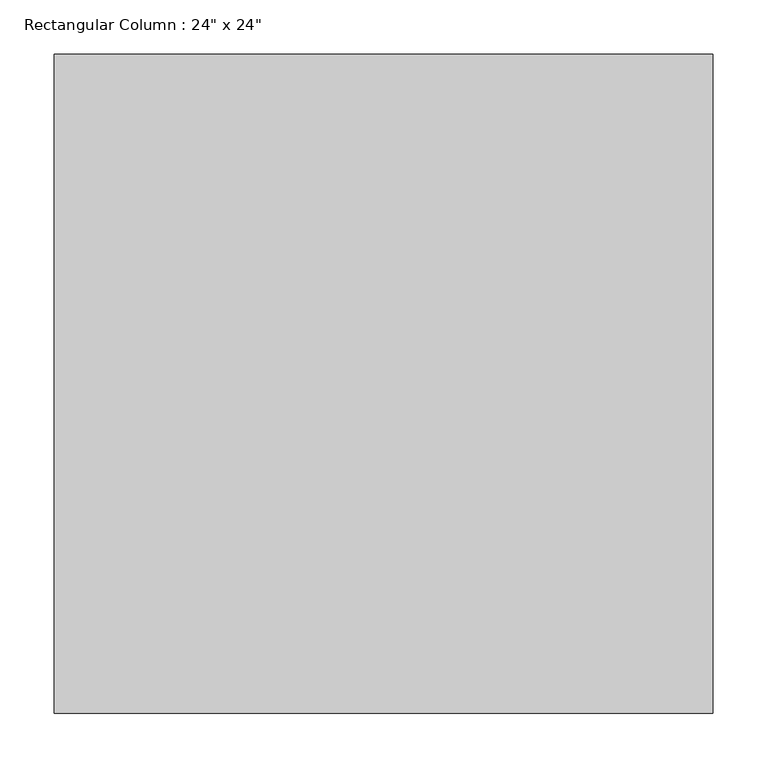
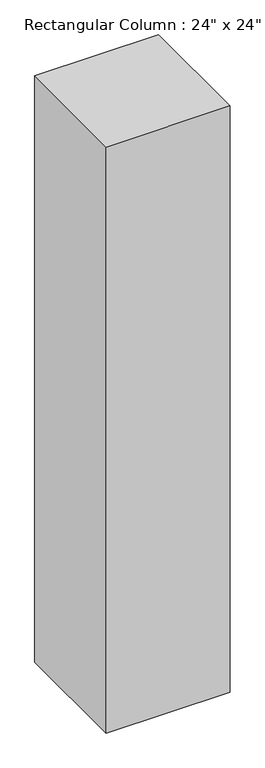
"""IFC4 building model written with IfcOpenShell, lengths in millimetres: column geometry."""

from ifc_helpers import new_model, si_unit, frame, origin, place, context, project, spatial, polyline, outline, extrude, source, transform, mapped, element, save


def column_ce31c9ba(model_context):
    return source(origin(), model_context, "Body", "SweptSolid", [
        extrude(outline(polyline([(304.8, 304.8), (304.8, -304.8), (-304.8, -304.8), (-304.8, 304.8), (304.8, 304.8)])), frame((0.0, 0.0, 6400.8), z_axis=(0.0, 0.0, 1.0), x_axis=(1.0, 0.0, 0.0)), (0.0, 0.0, 1.0), 3048.0),
    ])


if __name__ == "__main__":
    model = new_model("IFC4")
    model_context = context("Model", 3, world=origin())
    ifc_project = project(units=[si_unit("LENGTHUNIT", "METRE", prefix="MILLI")], contexts=[model_context])
    site = spatial("IfcSite", under=ifc_project)
    building = spatial("IfcBuilding", under=site)
    placement = place(None, origin())
    column_shape = column_ce31c9ba(model_context)
    element("IfcColumn", 1, ObjectType="Rectangular Column : 24\" x 24\"", at=placement, inside=building, context=model_context, shape_type="MappedRepresentation", body=[
        mapped(column_shape, transform((0.0, 0.0, 0.0), x_axis=(1.0, 0.0, 0.0), y_axis=(0.0, 1.0, 0.0), z_axis=(0.0, 0.0, 1.0))),
    ])
    save(model, "model.ifc")

# Revit data of these elements
# Type "Rectangular Column : 24\" x 24\""
#   Assembly Code = "B1010200"
#   Depth = 2' - 0"
#   Offset Base = 0' - 0"
#   Offset Top = 0' - 0"
#   Width = 2' - 0"
#   Material = none
